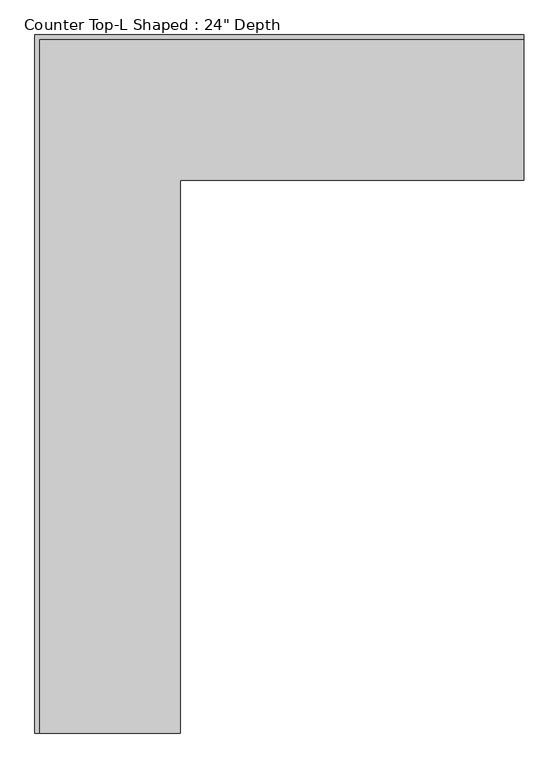
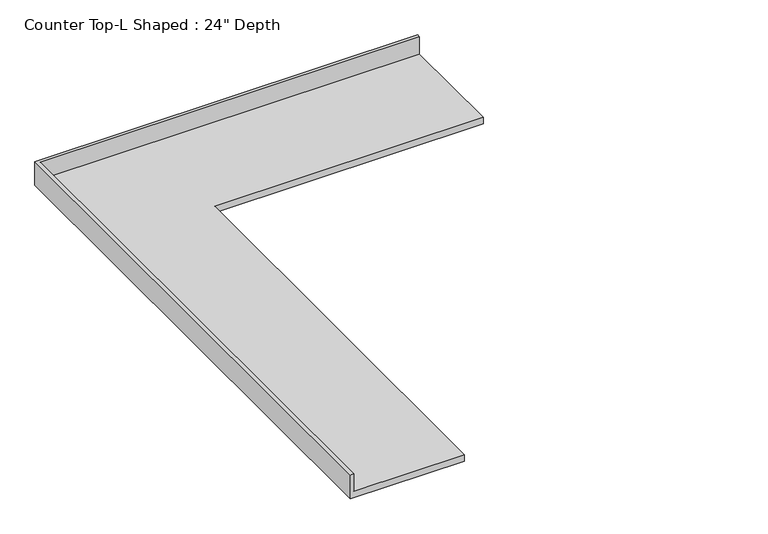
"""IFC4 building model written with IfcOpenShell, lengths in millimetres: furniture geometry."""

from ifc_helpers import new_model, si_unit, origin, place, context, project, spatial, faceted_brep, source, transform, mapped, element, save


def furniture_f5a42f9b(model_context):
    return source(origin(), model_context, "Body", "Brep", [
        faceted_brep([(-565.4622951, -3048.0, 914.4), (-565.4622951, -635.0, 914.4), (933.1377049, -635.0, 914.4), (933.1377049, -19.05, 914.4), (-1181.4122951, -19.05, 914.4), (-1181.4122951, -3048.0, 914.4), (933.1377049, 0.0, 876.3), (933.1377049, -635.0, 876.3), (-565.4622951, -635.0, 876.3), (-565.4622951, -3048.0, 876.3), (-1200.4622951, -3048.0, 876.3), (-1200.4622951, 0.0, 876.3), (-1200.4622951, 0.0, 1016.0), (933.1377049, 0.0, 1016.0), (-1200.4622951, -3048.0, 1016.0), (-1181.4122951, -3048.0, 1016.0), (933.1377049, -19.05, 1016.0), (-1181.4122951, -19.05, 1016.0)], [[[0, 1, 2, 3, 4, 5]], [[6, 7, 8, 9, 10, 11]], [[6, 11, 12, 13]], [[11, 10, 14, 12]], [[14, 10, 9, 0, 5, 15]], [[1, 0, 9, 8]], [[2, 1, 8, 7]], [[7, 6, 13, 16, 3, 2]], [[12, 14, 15, 17, 16, 13]], [[3, 16, 17, 4]], [[17, 15, 5, 4]]]),
    ])


if __name__ == "__main__":
    model = new_model("IFC4")
    model_context = context("Model", 3, world=origin())
    ifc_project = project(units=[si_unit("LENGTHUNIT", "METRE", prefix="MILLI")], contexts=[model_context])
    site = spatial("IfcSite", under=ifc_project)
    building = spatial("IfcBuilding", under=site)
    placement = place(None, origin())
    furniture_shape = furniture_f5a42f9b(model_context)
    element("IfcFurniture", 1, ObjectType="Counter Top-L Shaped : 24\" Depth", at=placement, inside=building, context=model_context, shape_type="MappedRepresentation", body=[
        mapped(furniture_shape, transform((0.0, 0.0, 0.0), x_axis=(1.0, 0.0, 0.0), y_axis=(0.0, 1.0, 0.0), z_axis=(0.0, 0.0, 1.0))),
    ])
    save(model, "model.ifc")

# Revit data of these elements
# Type "Counter Top-L Shaped : 24\" Depth"
#   Assembly Code = "C1030400"
#   Counter Thickness = 0' - 1 1/2"
#   Depth = 2' - 1"
#   Height = 3' - 0"
#   Length - Leg 1 [instance default] = 8' - 0"
#   Length - Leg 2 [instance default] = 6' - 0"
#   Counter Top Material = none
#   Default Elevation = 0
# Element 1 (IfcFurniture, "Counter Top-L Shaped : 24\" Depth")
#   Length - Leg 1 = 7' - 0"
#   Length - Leg 2 = 10' - 0"
#   Materials on its faces: "Counter Top"
# Materials
#   "Counter Top": class "Wood", colour RGB 226 177 128, transparency 0
